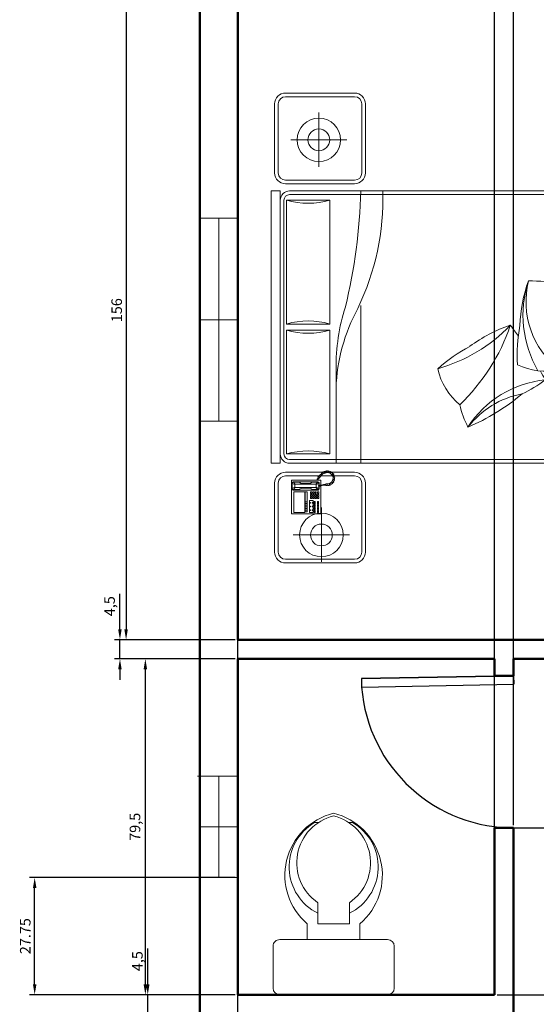
# Model space of a CAD drawing. Units: inches. Extents: x 907 to 2409, y 377 to 1163.
# Tile 4 of 9: x 936 to 1058, y 687 to 920. Entities that reach past the tile are written whole.
import ezdxf

# ---------------------------------------------------------------- set-up
doc = ezdxf.new("R2010")
doc.units = ezdxf.units.IN
for name, color, linetype, lineweight in [('A-ANNO-DIMS', 2, 'Continuous', 18), ('A-DOOR', 3, 'Continuous', 25), ('A-FLOR-FIXT', 9, 'Continuous', 18), ('A-FURN', 8, 'Continuous', 18), ('A-GLAZ', 4, 'Continuous', 18), ('A-WALL', 7, 'Continuous', 50)]:
    doc.layers.add(name, color=color, linetype=linetype, lineweight=lineweight)
doc.styles.get("Standard").update_dxf_attribs({"font": 'arial.ttf'})
doc.dimstyles.new('ISO-25', dxfattribs={"dimtxt": 2.5, "dimasz": 2.5, "dimexe": 1.25, "dimexo": 0.625, "dimtad": 1, "dimtxsty": 'Standard', "dimcen": 2.5, "dimadec": 0, "dimazin": 0, "dimtfac": 1, "dimtmove": 0, "dimatfit": 3, "dimfxl": 1, "dimarcsym": 0})

# ---------------------------------------------------------------- blocks, each defined once
blk = doc.blocks.new('A$C02F3725D')
for p, q in [((0.025, 0.69), (0.435, 0.69)), ((0, 0.505), (0, 0.665)), ((0.46, 0.665), (0.46, 0.505)), ((0.435, 0.48), (0.025, 0.48)), ((0.13, 0.48), (0.13, 0.42)), ((0.33, 0.42), (0.33, 0.48)), ((0.17, 0.34), (0.17, 0.42)), ((0.17, 0.42), (0.29, 0.42)), ((0.29, 0.34), (0.29, 0.42)), ((0.1578, 0.035), (0.1724, 0.035)), ((0.2876, 0.035), (0.3022, 0.035))]:
    blk.add_line(p, q)
for centre, radius, start, end in [((0.025, 0.665), 0.025, 90, 180), ((0.435, 0.665), 0.025, 0, 90), ((0.025, 0.505), 0.025, 180, 270), ((0.435, 0.505), 0.025, 270, 0), ((0.2874, 0.2356), 0.2425, 130.4885, 256.2965), ((0.1726, 0.2356), 0.2425, 283.7035, 49.5115), ((0.2568, 0.2042), 0.196, 116.2742, 239.6668), ((0.2032, 0.2042), 0.196, 300.3332, 63.7258), ((0.2732, 0.1883), 0.1834, 124.2157, 256.394), ((0.1868, 0.1883), 0.1834, 283.606, 55.7843)]:
    blk.add_arc(centre, radius, start, end)
blk = doc.blocks.new('A$C356F0359')
for p, q in [((0.4398, 1.9801), (0.0598, 1.9801)), ((0.4398, 1.9601), (0.0598, 1.9601)), ((0.5489, 2), (2.0492, 2)), ((0.5489, 1.9489), (0.5489, 2)), ((2.0492, 1.9489), (2.0492, 2)), ((2.5283, 1.9801), (2.1483, 1.9801)), ((2.5283, 1.9601), (2.1483, 1.9601)), ((-0.0002, 1.9201), (-0.0002, 1.5401)), ((0.0198, 1.9201), (0.0198, 1.5401)), ((0.4798, 1.5401), (0.4798, 1.9201)), ((0.4998, 1.5401), (0.4998, 1.9201)), ((2.0492, 1.9489), (0.5489, 1.9489)), ((1.998, 1.9289), (0.6001, 1.9289)), ((2.0883, 1.9201), (2.0883, 1.5401)), ((2.1083, 1.9201), (2.1083, 1.5401)), ((2.5683, 1.5401), (2.5683, 1.9201)), ((2.5883, 1.5401), (2.5883, 1.9201)), ((0.1539, 1.5681), (0.1539, 1.8777)), ((0.2725, 1.8879), (0.2702, 1.8856)), ((0.2702, 1.8856), (0.2702, 1.7279)), ((0.2725, 1.8879), (0.4531, 1.8879)), ((0.3913, 1.8753), (0.277, 1.8753)), ((0.277, 1.8753), (0.277, 1.8147)), ((0.3913, 1.8147), (0.3913, 1.8753)), ((0.4016, 1.8787), (0.4062, 1.8845)), ((0.4016, 1.7404), (0.4016, 1.8787)), ((0.4062, 1.881), (0.405, 1.8765)), ((0.405, 1.8765), (0.4153, 1.8662)), ((0.405, 1.8765), (0.405, 1.8456)), ((0.405, 1.8456), (0.4073, 1.8399)), ((0.4062, 1.8845), (0.4405, 1.8845)), ((0.4108, 1.8833), (0.4062, 1.881)), ((0.4108, 1.8833), (0.4382, 1.8833)), ((0.4165, 1.8685), (0.4108, 1.8833)), ((0.4153, 1.8662), (0.4165, 1.8685)), ((0.4153, 1.8147), (0.4153, 1.8662)), ((0.4325, 1.8685), (0.4165, 1.8685)), ((0.4325, 1.8685), (0.4382, 1.8833)), ((0.4336, 1.8662), (0.4325, 1.8685)), ((0.4439, 1.8765), (0.4336, 1.8662)), ((0.4336, 1.8147), (0.4336, 1.8662)), ((0.4382, 1.8833), (0.4428, 1.881)), ((0.4405, 1.8845), (0.4462, 1.8787)), ((0.4439, 1.8456), (0.4416, 1.8399)), ((0.4428, 1.881), (0.4439, 1.8765)), ((0.4439, 1.8765), (0.4439, 1.8456)), ((0.4462, 1.8787), (0.4462, 1.7416)), ((0.4531, 1.8879), (0.4553, 1.8856)), ((0.4553, 1.8856), (0.4553, 1.7279)), ((0.5489, 1.8977), (0.5489, 0.0512)), ((0.5689, 1.8977), (0.5689, 0.0512)), ((2.0292, 0.0512), (2.0292, 1.8977)), ((2.0492, 0.0512), (2.0492, 1.8977)), ((2.3306, 1.5822), (2.3306, 1.8917)), ((0.277, 1.8147), (0.3913, 1.8147)), ((0.3913, 1.8125), (0.2816, 1.8125)), ((0.2816, 1.8125), (0.2816, 1.801)), ((0.2816, 1.801), (0.3913, 1.801)), ((0.2907, 1.8125), (0.2907, 1.801)), ((0.2999, 1.8125), (0.2999, 1.801)), ((0.309, 1.8125), (0.309, 1.801)), ((0.3182, 1.8125), (0.3182, 1.801)), ((0.3273, 1.8125), (0.3273, 1.801)), ((0.3365, 1.8125), (0.3365, 1.801)), ((0.3913, 1.801), (0.3913, 1.8125)), ((0.4073, 1.8399), (0.4108, 1.8342)), ((0.4108, 1.8342), (0.4119, 1.8262)), ((0.4108, 1.785), (0.4119, 1.793)), ((0.4119, 1.8262), (0.4119, 1.8147)), ((0.4119, 1.793), (0.4119, 1.8147)), ((0.4153, 1.8147), (0.4153, 1.753)), ((0.4336, 1.8147), (0.4336, 1.753)), ((0.4382, 1.8342), (0.4371, 1.8262)), ((0.4371, 1.8262), (0.4371, 1.8147)), ((0.4371, 1.793), (0.4371, 1.8147)), ((0.4382, 1.785), (0.4371, 1.793)), ((0.4416, 1.8399), (0.4382, 1.8342)), ((0.277, 1.7885), (0.277, 1.7679)), ((0.3445, 1.7885), (0.277, 1.7885)), ((0.277, 1.7679), (0.3445, 1.7679)), ((0.2782, 1.7622), (0.2782, 1.7576)), ((0.2896, 1.7622), (0.2782, 1.7622)), ((0.2782, 1.7576), (0.2896, 1.7576)), ((0.2782, 1.745), (0.2896, 1.745)), ((0.2782, 1.7382), (0.2782, 1.745)), ((0.2896, 1.7382), (0.2782, 1.7382)), ((0.2885, 1.7862), (0.2885, 1.7827)), ((0.2919, 1.7862), (0.2885, 1.7862)), ((0.2885, 1.7827), (0.2919, 1.7827)), ((0.2919, 1.7736), (0.2885, 1.7736)), ((0.2885, 1.7736), (0.2885, 1.7702)), ((0.2885, 1.7702), (0.2919, 1.7702)), ((0.2896, 1.7576), (0.2896, 1.7622)), ((0.2896, 1.745), (0.2896, 1.7382)), ((0.2919, 1.7827), (0.2919, 1.7862)), ((0.2919, 1.7702), (0.2919, 1.7736)), ((0.2942, 1.7622), (0.2942, 1.7576)), ((0.3056, 1.7622), (0.2942, 1.7622)), ((0.2942, 1.7576), (0.3056, 1.7576)), ((0.2942, 1.745), (0.3056, 1.745)), ((0.2942, 1.7382), (0.2942, 1.745)), ((0.3056, 1.7382), (0.2942, 1.7382)), ((0.3056, 1.7576), (0.3056, 1.7622)), ((0.3056, 1.745), (0.3056, 1.7382)), ((0.3125, 1.7862), (0.309, 1.7862)), ((0.309, 1.7862), (0.309, 1.7827)), ((0.309, 1.7827), (0.3125, 1.7827)), ((0.3125, 1.7736), (0.309, 1.7736)), ((0.309, 1.7736), (0.309, 1.7702)), ((0.309, 1.7702), (0.3125, 1.7702)), ((0.3102, 1.7622), (0.3102, 1.7576)), ((0.3216, 1.7622), (0.3102, 1.7622)), ((0.3102, 1.7576), (0.3216, 1.7576)), ((0.3102, 1.745), (0.3216, 1.745)), ((0.3102, 1.7382), (0.3102, 1.745)), ((0.3216, 1.7382), (0.3102, 1.7382)), ((0.3125, 1.7827), (0.3125, 1.7862)), ((0.3125, 1.7702), (0.3125, 1.7736)), ((0.3216, 1.7576), (0.3216, 1.7622)), ((0.3216, 1.745), (0.3216, 1.7382)), ((0.3376, 1.7622), (0.3262, 1.7622)), ((0.3262, 1.7622), (0.3262, 1.7576)), ((0.3262, 1.7576), (0.3376, 1.7576)), ((0.3262, 1.7382), (0.3262, 1.745)), ((0.3262, 1.745), (0.3376, 1.745)), ((0.3376, 1.7382), (0.3262, 1.7382)), ((0.333, 1.7862), (0.3296, 1.7862)), ((0.3296, 1.7862), (0.3296, 1.7827)), ((0.3296, 1.7827), (0.333, 1.7827)), ((0.333, 1.7736), (0.3296, 1.7736)), ((0.3296, 1.7736), (0.3296, 1.7702)), ((0.3296, 1.7702), (0.333, 1.7702)), ((0.333, 1.7827), (0.333, 1.7862)), ((0.333, 1.7702), (0.333, 1.7736)), ((0.3376, 1.7576), (0.3376, 1.7622)), ((0.3376, 1.745), (0.3376, 1.7382)), ((0.3445, 1.7679), (0.3445, 1.7885)), ((0.3548, 1.7759), (0.3548, 1.7827)), ((0.3548, 1.7827), (0.3639, 1.7827)), ((0.3639, 1.7759), (0.3548, 1.7759)), ((0.3548, 1.7633), (0.3548, 1.7702)), ((0.3548, 1.7702), (0.3639, 1.7702)), ((0.3639, 1.7633), (0.3548, 1.7633)), ((0.3548, 1.7564), (0.3639, 1.7564)), ((0.3548, 1.7496), (0.3548, 1.7564)), ((0.3639, 1.7496), (0.3548, 1.7496)), ((0.3548, 1.737), (0.3548, 1.7439)), ((0.3548, 1.7439), (0.3639, 1.7439)), ((0.3639, 1.737), (0.3548, 1.737)), ((0.3639, 1.7827), (0.3639, 1.7759)), ((0.3639, 1.7702), (0.3639, 1.7633)), ((0.3639, 1.7564), (0.3639, 1.7496)), ((0.3639, 1.7439), (0.3639, 1.737)), ((0.3685, 1.7827), (0.3776, 1.7827)), ((0.3685, 1.7759), (0.3685, 1.7827)), ((0.3776, 1.7759), (0.3685, 1.7759)), ((0.3685, 1.7633), (0.3685, 1.7702)), ((0.3685, 1.7702), (0.3776, 1.7702)), ((0.3776, 1.7633), (0.3685, 1.7633)), ((0.3685, 1.7564), (0.3776, 1.7564)), ((0.3685, 1.7496), (0.3685, 1.7564)), ((0.3776, 1.7496), (0.3685, 1.7496)), ((0.3685, 1.737), (0.3685, 1.7439)), ((0.3685, 1.7439), (0.3776, 1.7439)), ((0.3776, 1.737), (0.3685, 1.737)), ((0.3776, 1.7827), (0.3776, 1.7759)), ((0.3776, 1.7702), (0.3776, 1.7633)), ((0.3776, 1.7564), (0.3776, 1.7496)), ((0.3776, 1.7439), (0.3776, 1.737)), ((0.3822, 1.7759), (0.3822, 1.7827)), ((0.3822, 1.7827), (0.3913, 1.7827)), ((0.3913, 1.7759), (0.3822, 1.7759)), ((0.3822, 1.7633), (0.3822, 1.7702)), ((0.3822, 1.7702), (0.3913, 1.7702)), ((0.3913, 1.7633), (0.3822, 1.7633)), ((0.3822, 1.7576), (0.3913, 1.7576)), ((0.3822, 1.7507), (0.3822, 1.7576)), ((0.3913, 1.7507), (0.3822, 1.7507)), ((0.3822, 1.7439), (0.3913, 1.7439)), ((0.3822, 1.737), (0.3822, 1.7439)), ((0.3913, 1.737), (0.3822, 1.737)), ((0.3913, 1.7827), (0.3913, 1.7759)), ((0.3913, 1.7702), (0.3913, 1.7633)), ((0.3913, 1.7576), (0.3913, 1.7507)), ((0.3913, 1.7439), (0.3913, 1.737)), ((0.4073, 1.7347), (0.4016, 1.7404)), ((0.405, 1.7736), (0.4073, 1.7793)), ((0.405, 1.7427), (0.405, 1.7736)), ((0.405, 1.7427), (0.4153, 1.753)), ((0.4062, 1.7382), (0.405, 1.7427)), ((0.4108, 1.7359), (0.4062, 1.7382)), ((0.4073, 1.7793), (0.4108, 1.785)), ((0.4165, 1.7507), (0.4108, 1.7359)), ((0.4108, 1.7359), (0.4234, 1.7359)), ((0.4153, 1.753), (0.4165, 1.7507)), ((0.4325, 1.7507), (0.4165, 1.7507)), ((0.4233, 1.7393), (0.4235, 1.7294)), ((0.4268, 1.7393), (0.4233, 1.7393)), ((0.4274, 1.7301), (0.4268, 1.7393)), ((0.427, 1.7359), (0.4382, 1.7359)), ((0.4336, 1.753), (0.4325, 1.7507)), ((0.4325, 1.7507), (0.4382, 1.7359)), ((0.4439, 1.7427), (0.4336, 1.753)), ((0.4416, 1.7793), (0.4382, 1.785)), ((0.4382, 1.7359), (0.4428, 1.7382)), ((0.4462, 1.7416), (0.4405, 1.7347)), ((0.4439, 1.7736), (0.4416, 1.7793)), ((0.4428, 1.7382), (0.4439, 1.7427)), ((0.4439, 1.7427), (0.4439, 1.7736)), ((0.4622, 1.7459), (0.4553, 1.7484)), ((0.4553, 1.7439), (0.4604, 1.7425)), ((0.4604, 1.7425), (0.465, 1.7388)), ((0.4654, 1.7427), (0.4622, 1.7459)), ((0.465, 1.7388), (0.4662, 1.7372)), ((0.4678, 1.7405), (0.4654, 1.7427)), ((0.4662, 1.7372), (0.4686, 1.7374)), ((0.4686, 1.7374), (0.4662, 1.735)), ((0.4721, 1.7421), (0.4678, 1.7405)), ((0.4741, 1.7401), (0.4721, 1.7421)), ((0.4725, 1.7366), (0.4741, 1.7401)), ((0.4753, 1.7388), (0.4725, 1.7366)), ((0.4783, 1.7356), (0.4753, 1.7388)), ((2.4819, 1.7366), (2.1818, 1.7366)), ((0.3052, 1.7226), (0.0051, 1.7226)), ((0.2702, 1.7279), (0.2725, 1.7256)), ((0.4244, 1.7256), (0.2725, 1.7256)), ((0.4234, 1.7347), (0.4073, 1.7347)), ((0.4235, 1.7294), (0.4263, 1.7179)), ((0.4263, 1.7179), (0.429, 1.707)), ((0.427, 1.697), (0.4265, 1.6915)), ((0.4265, 1.6915), (0.4332, 1.6903)), ((0.4332, 1.6903), (0.4267, 1.6864)), ((0.4267, 1.6864), (0.4272, 1.6801)), ((0.4295, 1.6996), (0.427, 1.697)), ((0.4405, 1.7347), (0.4271, 1.7347)), ((0.429, 1.7227), (0.4274, 1.7301)), ((0.4531, 1.7256), (0.4284, 1.7256)), ((0.429, 1.707), (0.4288, 1.701)), ((0.4288, 1.701), (0.4295, 1.6996)), ((0.4318, 1.7119), (0.429, 1.7227)), ((0.4325, 1.7063), (0.4318, 1.7119)), ((0.4323, 1.7003), (0.4325, 1.7063)), ((0.4364, 1.6973), (0.4323, 1.7003)), ((0.4355, 1.6919), (0.4364, 1.6973)), ((0.4367, 1.6774), (0.4355, 1.6919)), ((0.4553, 1.7279), (0.4531, 1.7256)), ((0.4662, 1.735), (0.4755, 1.7268)), ((0.4755, 1.7268), (0.4906, 1.7139)), ((0.4759, 1.729), (0.4783, 1.7356)), ((0.4821, 1.7322), (0.4759, 1.729)), ((0.4874, 1.7272), (0.4821, 1.7322)), ((0.4862, 1.7199), (0.4874, 1.7272)), ((0.4914, 1.7231), (0.4862, 1.7199)), ((0.4908, 1.7135), (0.4984, 1.6917)), ((0.4958, 1.7185), (0.4914, 1.7231)), ((0.494, 1.7135), (0.4958, 1.7185)), ((0.501, 1.7142), (0.494, 1.7135)), ((0.4984, 1.6917), (0.4952, 1.6744)), ((0.4964, 1.7047), (0.5031, 1.7072)), ((0.5038, 1.7049), (0.4964, 1.7047)), ((0.5005, 1.695), (0.5054, 1.6996)), ((0.5068, 1.695), (0.5005, 1.695)), ((0.5008, 1.6871), (0.5079, 1.6892)), ((0.5068, 1.6836), (0.5008, 1.6871)), ((0.5031, 1.7072), (0.501, 1.7142)), ((0.5054, 1.6996), (0.5038, 1.7049)), ((0.5058, 1.679), (0.5068, 1.6836)), ((0.5079, 1.6892), (0.5068, 1.695)), ((0.4272, 1.6801), (0.4346, 1.6794)), ((0.4346, 1.6794), (0.4281, 1.6744)), ((0.4281, 1.6744), (0.4311, 1.669)), ((0.4311, 1.669), (0.4381, 1.6704)), ((0.4381, 1.6704), (0.4348, 1.6639)), ((0.4348, 1.6639), (0.4383, 1.6598)), ((0.4455, 1.6663), (0.4367, 1.6774)), ((0.4383, 1.6598), (0.4436, 1.6637)), ((0.4436, 1.6637), (0.4427, 1.6575)), ((0.4427, 1.6575), (0.4471, 1.6547)), ((0.4577, 1.6598), (0.4455, 1.6663)), ((0.4471, 1.6547), (0.4526, 1.6593)), ((0.4526, 1.6593), (0.4519, 1.6517)), ((0.4519, 1.6517), (0.4568, 1.6503)), ((0.4568, 1.6503), (0.4598, 1.6565)), ((0.4716, 1.6586), (0.4577, 1.6598)), ((0.4598, 1.6565), (0.4626, 1.6503)), ((0.4626, 1.6503), (0.4665, 1.6498)), ((0.4665, 1.6498), (0.4681, 1.6565)), ((0.4681, 1.6565), (0.4707, 1.6491)), ((0.4707, 1.6491), (0.4751, 1.6503)), ((0.485, 1.6644), (0.4716, 1.6586)), ((0.4751, 1.6503), (0.4753, 1.6565)), ((0.4753, 1.6565), (0.4806, 1.6519)), ((0.4806, 1.6519), (0.4843, 1.6538)), ((0.4843, 1.6538), (0.4836, 1.6607)), ((0.4836, 1.6607), (0.4885, 1.6547)), ((0.4952, 1.6744), (0.485, 1.6644)), ((0.4885, 1.6547), (0.4922, 1.6579)), ((0.4922, 1.6579), (0.4894, 1.6642)), ((0.4894, 1.6642), (0.4959, 1.6614)), ((0.4957, 1.6704), (0.5024, 1.6683)), ((0.4989, 1.6642), (0.4957, 1.6704)), ((0.4959, 1.6614), (0.4989, 1.6642)), ((0.5042, 1.673), (0.4987, 1.6792)), ((0.4987, 1.6792), (0.5058, 1.679)), ((0.5024, 1.6683), (0.5042, 1.673)), ((0.0598, 1.5001), (0.4398, 1.5001)), ((0.0598, 1.4801), (0.4398, 1.4801)), ((2.1483, 1.5001), (2.5283, 1.5001)), ((2.1483, 1.4801), (2.5283, 1.4801)), ((0.6001, 0.02), (1.998, 0.02)), ((0.6001, 0), (1.998, 0))]:
    blk.add_line(p, q)
at = {"linetype": 'ByBlock'}
for p, q in [((0.6001, 1.9147), (1.282, 1.9147)), ((0.6001, 1.6759), (0.6001, 1.9147)), ((1.282, 1.9147), (1.282, 1.6759)), ((1.3161, 1.9147), (1.998, 1.9147)), ((1.3161, 1.6759), (1.3161, 1.9147)), ((1.998, 1.9147), (1.998, 1.6759)), ((1.0687, 1.6418), (0.5489, 1.6418)), ((1.282, 1.6759), (0.6001, 1.6759)), ((1.998, 1.6759), (1.3161, 1.6759)), ((1.4185, 1.5053), (0.5489, 1.5053))]:
    blk.add_line(p, q, dxfattribs=at)
for centre in [(2.3306, 1.7366), (0.1539, 1.7226)]:
    blk.add_circle(centre, 0.12, dxfattribs=at)
for centre in [(2.3306, 1.7366), (0.1539, 1.7226)]:
    blk.add_circle(centre, 0.06)
for centre, radius, start, end in [((0.0598, 1.9201), 0.06, 90, 180), ((0.0598, 1.9201), 0.04, 90, 180), ((0.4398, 1.9201), 0.06, 0, 90), ((0.4398, 1.9201), 0.04, 0, 90), ((2.1483, 1.9201), 0.06, 90, 180), ((2.1483, 1.9201), 0.04, 90, 180), ((2.5283, 1.9201), 0.06, 0, 90), ((2.5283, 1.9201), 0.04, 0, 90), ((0.6001, 1.8977), 0.0512, 90, 180), ((0.6001, 1.8977), 0.0312, 90, 180), ((1.998, 1.8977), 0.0512, 0, 90), ((1.998, 1.8977), 0.0312, 0, 90), ((0.0598, 1.5401), 0.06, 180, 270), ((0.0598, 1.5401), 0.04, 180, 270), ((0.4398, 1.5401), 0.04, 270, 0), ((0.4398, 1.5401), 0.06, 270, 0), ((2.1483, 1.5401), 0.06, 180, 270), ((2.1483, 1.5401), 0.04, 180, 270), ((2.5283, 1.5401), 0.06, 270, 0), ((2.5283, 1.5401), 0.04, 270, 0), ((1.1471, 0.7332), 0.3575, 102.4782, 140.4625), ((1.9086, 1.3124), 0.8697, 195.336, 226.4193), ((0.3249, 0.4335), 0.9879, 28.4971, 41.0566), ((0.9965, 0.4273), 0.548, 103.2034, 117.0362), ((1.6529, 1.7059), 1.0798, 223.6306, 251.4288), ((0.4451, 0.4375), 0.5655, 5.3391, 57.6895), ((0.4517, 0.5274), 0.4879, 10.6986, 52.6864), ((1.8195, 1.3719), 1.1652, 203.0642, 220.3209), ((0.5617, 0.4344), 0.7874, 18.3527, 36.6851), ((-0.021, 2.4319), 2.1977, 305.2966, 307.2418), ((1.5949, 0.9312), 0.734, 205.259, 216.9351), ((1.4135, 0.487), 0.3575, 154.0418, 192.0262), ((1.3641, 0.0041), 0.6085, 71.81, 120.1351), ((1.1372, -0.3434), 0.9879, 80.0607, 92.6202), ((1.2836, -0.1573), 0.7874, 69.9163, 88.2487), ((1.44, 0.1186), 0.4774, 76.1849, 142.0017), ((-0.6432, 0.628), 2.1977, 349.4884, 358.8054), ((-0.021, 2.4319), 2.1977, 297.9248, 299.3793), ((1.5595, 0.1789), 0.548, 154.767, 168.5998), ((1.2647, 0.9578), 0.6885, 250.2936, 293.6414), ((1.3312, 1.4107), 1.1652, 254.6278, 271.8845), ((1.5368, 0.9609), 0.734, 256.8226, 268.4988), ((0.5943, 0.0454), 0.0458, 172.7599, 277.2401), ((0.5943, 0.0454), 0.0258, 172.7599, 277.2401), ((2.0038, 0.0454), 0.0458, 262.7599, 7.2401), ((2.0038, 0.0454), 0.0258, 262.7599, 7.2401)]:
    blk.add_arc(centre, radius, start, end)
for centre, radius, start, end in [((0.1906, 1.7953), 0.4265, 343.7398, 16.2602), ((1.6914, 1.7953), 0.4265, 163.7398, 196.2602), ((0.9067, 1.7953), 0.4265, 343.7398, 16.2602), ((2.4075, 1.7953), 0.4265, 163.7398, 196.2602), ((0.9303, 0.657), 0.9853, 61.4328, 88.1261), ((1.0826, 0.5712), 1.0706, 72.1966, 90.7418), ((2.1368, 4.5996), 3.0955, 256.4201, 268.3789), ((2.0056, 2.7745), 1.3903, 244.2427, 271.7984)]:
    blk.add_arc(centre, radius, start, end, dxfattribs=at)
blk = doc.blocks.new('*D31')
at = {"layer": 'A-ANNO-DIMS', "color": 0, "lineweight": -2, "transparency": 16777216}
for p, q in [((986.99, 929.12), (959.95, 929.12)), ((961.2, 926.62), (961.2, 775.62)), ((986.99, 773.12), (959.95, 773.12))]:
    blk.add_line(p, q, dxfattribs=at)
at = {"layer": 'A-ANNO-DIMS', "color": 0, "transparency": 16777216}
for points in [[(960.78, 926.62), (961.62, 926.62), (961.2, 929.12)], [(960.78, 775.62), (961.62, 775.62), (961.2, 773.12)]]:
    blk.add_solid(points, dxfattribs=at)
at = {"layer": 'Defpoints', "color": 0, "transparency": 16777216}
for p in [(987.61, 929.12), (961.2, 773.12), (987.61, 773.12)]:
    blk.add_point(p, dxfattribs=at)
at = {"layer": 'A-ANNO-DIMS', "color": 0, "transparency": 16777216, "insert": (959.3, 851.12), "char_height": 2.5, "attachment_point": 5, "rotation": 90}
blk.add_mtext('156', dxfattribs=at)
blk = doc.blocks.new('*D32')
at = {"layer": 'A-ANNO-DIMS', "color": 0, "lineweight": -2, "transparency": 16777216}
for p, q in [((959.75, 775.62), (959.75, 784.04)), ((986.99, 773.12), (958.5, 773.12)), ((959.75, 768.62), (959.75, 773.12)), ((986.99, 768.62), (958.5, 768.62)), ((959.75, 766.12), (959.75, 763.62))]:
    blk.add_line(p, q, dxfattribs=at)
at = {"layer": 'A-ANNO-DIMS', "color": 0, "transparency": 16777216}
for points in [[(959.33, 775.62), (960.16, 775.62), (959.75, 773.12)], [(959.33, 766.12), (960.16, 766.12), (959.75, 768.62)]]:
    blk.add_solid(points, dxfattribs=at)
at = {"layer": 'Defpoints', "color": 0, "transparency": 16777216}
for p in [(959.75, 773.12), (987.61, 773.12), (987.61, 768.62)]:
    blk.add_point(p, dxfattribs=at)
at = {"layer": 'A-ANNO-DIMS', "color": 0, "transparency": 16777216, "insert": (957.62, 781.08), "char_height": 2.5, "attachment_point": 5, "rotation": 90}
blk.add_mtext('4,5', dxfattribs=at)
blk = doc.blocks.new('*D33')
at = {"layer": 'A-ANNO-DIMS', "color": 0, "lineweight": -2, "transparency": 16777216}
for p, q in [((986.99, 768.62), (964.51, 768.62)), ((965.76, 691.62), (965.76, 766.12)), ((986.99, 689.12), (964.51, 689.12))]:
    blk.add_line(p, q, dxfattribs=at)
at = {"layer": 'A-ANNO-DIMS', "color": 0, "transparency": 16777216}
for points in [[(965.34, 766.12), (966.17, 766.12), (965.76, 768.62)], [(965.34, 691.62), (966.17, 691.62), (965.76, 689.12)]]:
    blk.add_solid(points, dxfattribs=at)
at = {"layer": 'Defpoints', "color": 0, "transparency": 16777216}
for p in [(965.76, 768.62), (987.61, 768.62), (987.61, 689.12)]:
    blk.add_point(p, dxfattribs=at)
at = {"layer": 'A-ANNO-DIMS', "color": 0, "transparency": 16777216, "insert": (963.63, 728.87), "char_height": 2.5, "attachment_point": 5, "rotation": 90}
blk.add_mtext('79,5', dxfattribs=at)
blk = doc.blocks.new('*D34')
at = {"layer": 'A-ANNO-DIMS', "color": 0, "lineweight": -2, "transparency": 16777216}
for p, q in [((966.32, 691.62), (966.32, 700.04)), ((986.99, 689.12), (965.07, 689.12)), ((966.32, 684.62), (966.32, 689.12)), ((986.99, 684.62), (965.07, 684.62)), ((966.32, 682.12), (966.32, 679.62))]:
    blk.add_line(p, q, dxfattribs=at)
at = {"layer": 'A-ANNO-DIMS', "color": 0, "transparency": 16777216}
for points in [[(965.9, 691.62), (966.74, 691.62), (966.32, 689.12)], [(965.9, 682.12), (966.74, 682.12), (966.32, 684.62)]]:
    blk.add_solid(points, dxfattribs=at)
at = {"layer": 'Defpoints', "color": 0, "transparency": 16777216}
for p in [(966.32, 689.12), (987.61, 689.12), (987.61, 684.62)]:
    blk.add_point(p, dxfattribs=at)
at = {"layer": 'A-ANNO-DIMS', "color": 0, "transparency": 16777216, "insert": (964.2, 697.08), "char_height": 2.5, "attachment_point": 5, "rotation": 90}
blk.add_mtext('4,5', dxfattribs=at)
blk = doc.blocks.new('DOOR-36IN')
for p, q in [((36, 36), (36, 0)), ((36, 0), (34, 0)), ((36, 0), (34, 0))]:
    blk.add_line(p, q)
blk.add_lwpolyline([(36, 36), (34, 36), (34, 0), (36, 0)], close=True)
blk.add_arc((36.06, 0), 36.06, 93.2732, 180)
blk = doc.blocks.new('WIN-24IN')
for p, q in [((0.53, 23.99), (0, 23.99)), ((9.53, 24), (0.53, 24)), ((5.03, 0), (5.03, 24)), ((9.53, 12), (0.53, 12)), ((9.53, 0), (0.53, 0))]:
    blk.add_line(p, q)
blk = doc.blocks.new('WIN-48IN')
for p, q in [((9, 48), (0, 48)), ((4.5, 48), (4.5, 0)), ((9, 24), (0, 24)), ((9, 0), (0, 0))]:
    blk.add_line(p, q)
blk = doc.blocks.new('*D59')
at = {"layer": 'A-ANNO-DIMS', "color": 0, "lineweight": -2, "transparency": 16777216}
for p, q in [((987.61, 773.75), (987.61, 1056.62)), ((1156.36, 773.75), (1156.36, 1056.62)), ((990.11, 1055.37), (1153.86, 1055.37))]:
    blk.add_line(p, q, dxfattribs=at)
at = {"layer": 'A-ANNO-DIMS', "color": 0, "transparency": 16777216}
for points in [[(990.11, 1055.79), (990.11, 1054.95), (987.61, 1055.37)], [(1153.86, 1055.79), (1153.86, 1054.95), (1156.36, 1055.37)]]:
    blk.add_solid(points, dxfattribs=at)
at = {"layer": 'Defpoints', "color": 0, "transparency": 16777216}
for p in [(1156.36, 1055.37), (987.61, 773.12), (1156.36, 773.12)]:
    blk.add_point(p, dxfattribs=at)
at = {"layer": 'A-ANNO-DIMS', "color": 0, "transparency": 16777216, "insert": (1071.99, 1057.27), "char_height": 2.5, "attachment_point": 5}
blk.add_mtext('168.75', dxfattribs=at)
blk = doc.blocks.new('*D60')
at = {"layer": 'A-ANNO-DIMS', "color": 0, "lineweight": -2, "transparency": 16777216}
for p, q in [((987.61, 689.75), (987.61, 1056.62)), ((1048.36, 689.75), (1048.36, 1056.62)), ((990.11, 1055.37), (1045.86, 1055.37))]:
    blk.add_line(p, q, dxfattribs=at)
at = {"layer": 'A-ANNO-DIMS', "color": 0, "transparency": 16777216}
for points in [[(990.11, 1055.79), (990.11, 1054.95), (987.61, 1055.37)], [(1045.86, 1055.79), (1045.86, 1054.95), (1048.36, 1055.37)]]:
    blk.add_solid(points, dxfattribs=at)
at = {"layer": 'Defpoints', "color": 0, "transparency": 16777216}
for p in [(1048.36, 1055.37), (987.61, 689.12), (1048.36, 689.12)]:
    blk.add_point(p, dxfattribs=at)
at = {"layer": 'A-ANNO-DIMS', "color": 0, "transparency": 16777216, "insert": (1017.99, 1057.27), "char_height": 2.5, "attachment_point": 5}
blk.add_mtext('60.75', dxfattribs=at)
blk = doc.blocks.new('*D61')
at = {"layer": 'A-ANNO-DIMS', "color": 0, "lineweight": -2, "transparency": 16777216}
for p, q in [((1052.86, 729.25), (1052.86, 1056.62)), ((1196.86, 727.25), (1196.86, 1056.62)), ((1055.36, 1055.37), (1194.36, 1055.37))]:
    blk.add_line(p, q, dxfattribs=at)
at = {"layer": 'A-ANNO-DIMS', "color": 0, "transparency": 16777216}
for points in [[(1055.36, 1055.79), (1055.36, 1054.95), (1052.86, 1055.37)], [(1194.36, 1055.79), (1194.36, 1054.95), (1196.86, 1055.37)]]:
    blk.add_solid(points, dxfattribs=at)
at = {"layer": 'Defpoints', "color": 0, "transparency": 16777216}
for p in [(1196.86, 1055.37), (1052.86, 728.62), (1196.86, 726.62)]:
    blk.add_point(p, dxfattribs=at)
at = {"layer": 'A-ANNO-DIMS', "color": 0, "transparency": 16777216, "insert": (1124.86, 1057.25), "char_height": 2.5, "attachment_point": 5}
blk.add_mtext('144', dxfattribs=at)
blk = doc.blocks.new('*D62')
at = {"layer": 'A-ANNO-DIMS', "color": 0, "lineweight": -2, "transparency": 16777216}
for p, q in [((987.61, 426.5), (987.61, 1056.62)), ((1096.36, 426.5), (1096.36, 1056.62)), ((990.11, 1055.37), (1093.86, 1055.37))]:
    blk.add_line(p, q, dxfattribs=at)
at = {"layer": 'A-ANNO-DIMS', "color": 0, "transparency": 16777216}
for points in [[(990.11, 1055.79), (990.11, 1054.95), (987.61, 1055.37)], [(1093.86, 1055.79), (1093.86, 1054.95), (1096.36, 1055.37)]]:
    blk.add_solid(points, dxfattribs=at)
at = {"layer": 'Defpoints', "color": 0, "transparency": 16777216}
for p in [(1096.36, 1055.37), (987.61, 425.87), (1096.36, 425.87)]:
    blk.add_point(p, dxfattribs=at)
at = {"layer": 'A-ANNO-DIMS', "color": 0, "transparency": 16777216, "insert": (1041.99, 1057.27), "char_height": 2.5, "attachment_point": 5}
blk.add_mtext('108.75', dxfattribs=at)
blk = doc.blocks.new('*D71')
at = {"layer": 'A-ANNO-DIMS', "color": 0, "lineweight": -2, "transparency": 16777216}
for p, q in [((986.99, 716.87), (938.33, 716.87)), ((939.58, 691.62), (939.58, 714.37)), ((986.99, 689.12), (938.33, 689.12))]:
    blk.add_line(p, q, dxfattribs=at)
at = {"layer": 'A-ANNO-DIMS', "color": 0, "transparency": 16777216}
for points in [[(939.17, 714.37), (940, 714.37), (939.58, 716.87)], [(939.17, 691.62), (940, 691.62), (939.58, 689.12)]]:
    blk.add_solid(points, dxfattribs=at)
at = {"layer": 'Defpoints', "color": 0, "transparency": 16777216}
for p in [(939.58, 716.87), (987.61, 716.87), (987.61, 689.12)]:
    blk.add_point(p, dxfattribs=at)
at = {"layer": 'A-ANNO-DIMS', "color": 0, "transparency": 16777216, "insert": (937.68, 703), "char_height": 2.5, "attachment_point": 5, "rotation": 90}
blk.add_mtext('27.75', dxfattribs=at)
blk = doc.blocks.new('*D81')
at = {"layer": 'A-ANNO-DIMS', "color": 0, "lineweight": -2, "transparency": 16777216}
for p, q in [((1053.49, 728.62), (1378.36, 728.62)), ((1377.11, 726.12), (1377.11, 691.62)), ((1048.99, 689.12), (1378.36, 689.12))]:
    blk.add_line(p, q, dxfattribs=at)
at = {"layer": 'A-ANNO-DIMS', "color": 0, "transparency": 16777216}
for points in [[(1376.7, 726.12), (1377.53, 726.12), (1377.11, 728.62)], [(1376.7, 691.62), (1377.53, 691.62), (1377.11, 689.12)]]:
    blk.add_solid(points, dxfattribs=at)
at = {"layer": 'Defpoints', "color": 0, "transparency": 16777216}
for p in [(1052.86, 728.62), (1048.36, 689.12), (1377.11, 689.12)]:
    blk.add_point(p, dxfattribs=at)
at = {"layer": 'A-ANNO-DIMS', "color": 0, "transparency": 16777216, "insert": (1375.21, 708.87), "char_height": 2.5, "attachment_point": 5, "rotation": 90}
blk.add_mtext('39.5', dxfattribs=at)

msp = doc.modelspace()

# ---------------------------------------------------------------- linework, layer by layer
at = {"layer": 'A-WALL'}
for p, q in [((978.6122, 1016.8705), (978.6122, 416.8705)), ((978.6122, 926.8705), (978.6122, 770.8705)), ((987.6122, 924.6205), (987.6122, 773.1205)), ((987.6122, 773.1205), (1116.3622, 773.1205)), ((987.6122, 768.6205), (1048.3622, 768.6205)), ((987.6122, 768.6205), (987.6122, 689.1205)), ((1048.3622, 768.6205), (1048.3622, 764.6205)), ((1052.8622, 768.6205), (1052.8622, 764.6205)), ((1052.8622, 768.6205), (1116.3622, 768.6205)), ((1048.3622, 764.6205), (1052.8622, 764.6205)), ((1048.3622, 728.6205), (1052.8622, 728.6205)), ((1048.3622, 728.6205), (1048.3622, 689.1205)), ((1052.8622, 728.6205), (1052.8622, 617.1205)), ((987.6122, 689.1205), (1048.3622, 689.1205))]:
    msp.add_line(p, q, dxfattribs=at)
msp.add_lwpolyline([(1216.3622, 416.8705), (1338.6122, 416.8705), (1338.6122, 1016.8705), (978.6122, 1016.8705), (978.6122, 416.8705), (1100.8622, 416.8705)], dxfattribs=at)

# ---------------------------------------------------------------- block references
at = {"layer": 'A-DOOR', "rotation": 91.08740474419501}
msp.add_blockref('DOOR-36IN', (1053.5454, 728.627), dxfattribs=at)
at = {"layer": 'A-FLOR-FIXT', "xscale": 62.24890487658392, "yscale": 62.24890487658392, "zscale": 62.24890487658392, "rotation": 180}
msp.add_blockref('A$C02F3725D', (1024.6094, 732.0723), dxfattribs=at)
at = {"layer": 'A-FURN', "xscale": 42.95257138859579, "yscale": 42.95257138859579, "zscale": 42.95257138859579, "rotation": 90}
msp.add_blockref('A$C356F0359', (1081.3864, 791.3196), dxfattribs=at)
at = {"layer": 'A-GLAZ'}
for name, p in [('WIN-48IN', (978.612, 824.871)), ('WIN-24IN', (978.083, 716.871))]:
    msp.add_blockref(name, p, dxfattribs=at)

# ---------------------------------------------------------------- dimensions: what is measured, and where the dimension line sits
at = {"layer": 'A-ANNO-DIMS'}
for base, p1, p2, override, picture, middle in [((1156.3622, 1055.3705), (987.6122, 773.1205), (1156.3622, 773.1205), {"dimdec": 2, "dimlfac": 1, "dimrnd": 0, "dimzin": 0, "dimdsep": 46, "dimlunit": 2}, '*D59', (1071.9872, 1057.272)), ((1048.3622, 1055.3705), (987.6122, 689.1205), (1048.3622, 689.1205), {"dimdec": 2, "dimlfac": 1, "dimrnd": 0, "dimzin": 0, "dimdsep": 46, "dimlunit": 2}, '*D60', (1017.9872, 1057.272)), ((1096.3622, 1055.3705), (987.6122, 425.8705), (1096.3622, 425.8705), {"dimdec": 2, "dimlfac": 1, "dimrnd": 0, "dimzin": 0, "dimdsep": 46, "dimlunit": 2}, '*D62', (1041.9872, 1057.272)), ((1196.8622, 1055.3705), (1052.8622, 728.6205), (1196.8622, 726.6205), {"dimdec": 0, "dimlfac": 1, "dimrnd": 0, "dimzin": 0, "dimdsep": 46, "dimlunit": 2}, '*D61', (1124.8622, 1057.2507))]:
    dim = msp.add_linear_dim(base=base, p1=p1, p2=p2, dimstyle='ISO-25', override=override, dxfattribs=at)
    dim.commit()
    dim.dimension.update_dxf_attribs({"geometry": picture, "text_midpoint": middle})
for base, p1, p2, override, picture, middle in [((961.1988, 773.1205), (987.6122, 929.1205), (987.6122, 773.1205), {"dimclrd": 0, "dimclre": 0, "dimclrt": 0}, '*D31', (959.2973, 851.1205)), ((959.7452, 773.1205), (987.6122, 768.6205), (987.6122, 773.1205), {"dimclrd": 0, "dimclre": 0, "dimclrt": 0}, '*D32', (957.6229, 781.081)), ((965.7575, 768.6205), (987.6122, 689.1205), (987.6122, 768.6205), {"dimclrd": 0, "dimclre": 0, "dimclrt": 0}, '*D33', (963.6301, 728.8705)), ((1377.1122, 689.1205), (1052.8622, 728.6205), (1048.3622, 689.1205), {"dimdec": 1, "dimlfac": 1, "dimrnd": 0, "dimzin": 0, "dimdsep": 46, "dimlunit": 2}, '*D81', (1375.2099, 708.8705)), ((939.5829, 716.8705), (987.6122, 689.1205), (987.6122, 716.8705), {"dimdec": 2, "dimlfac": 1, "dimrnd": 0, "dimzin": 0, "dimdsep": 46, "dimlunit": 2}, '*D71', (937.6815, 702.9955)), ((966.319, 689.1205), (987.6122, 684.6205), (987.6122, 689.1205), {"dimclrd": 0, "dimclre": 0, "dimclrt": 0}, '*D34', (964.1967, 697.081))]:
    dim = msp.add_linear_dim(base=base, p1=p1, p2=p2, angle=90, dimstyle='ISO-25', override=override, dxfattribs=at)
    dim.commit()
    dim.dimension.update_dxf_attribs({"geometry": picture, "text_midpoint": middle})

doc.saveas('drawing.dxf')
